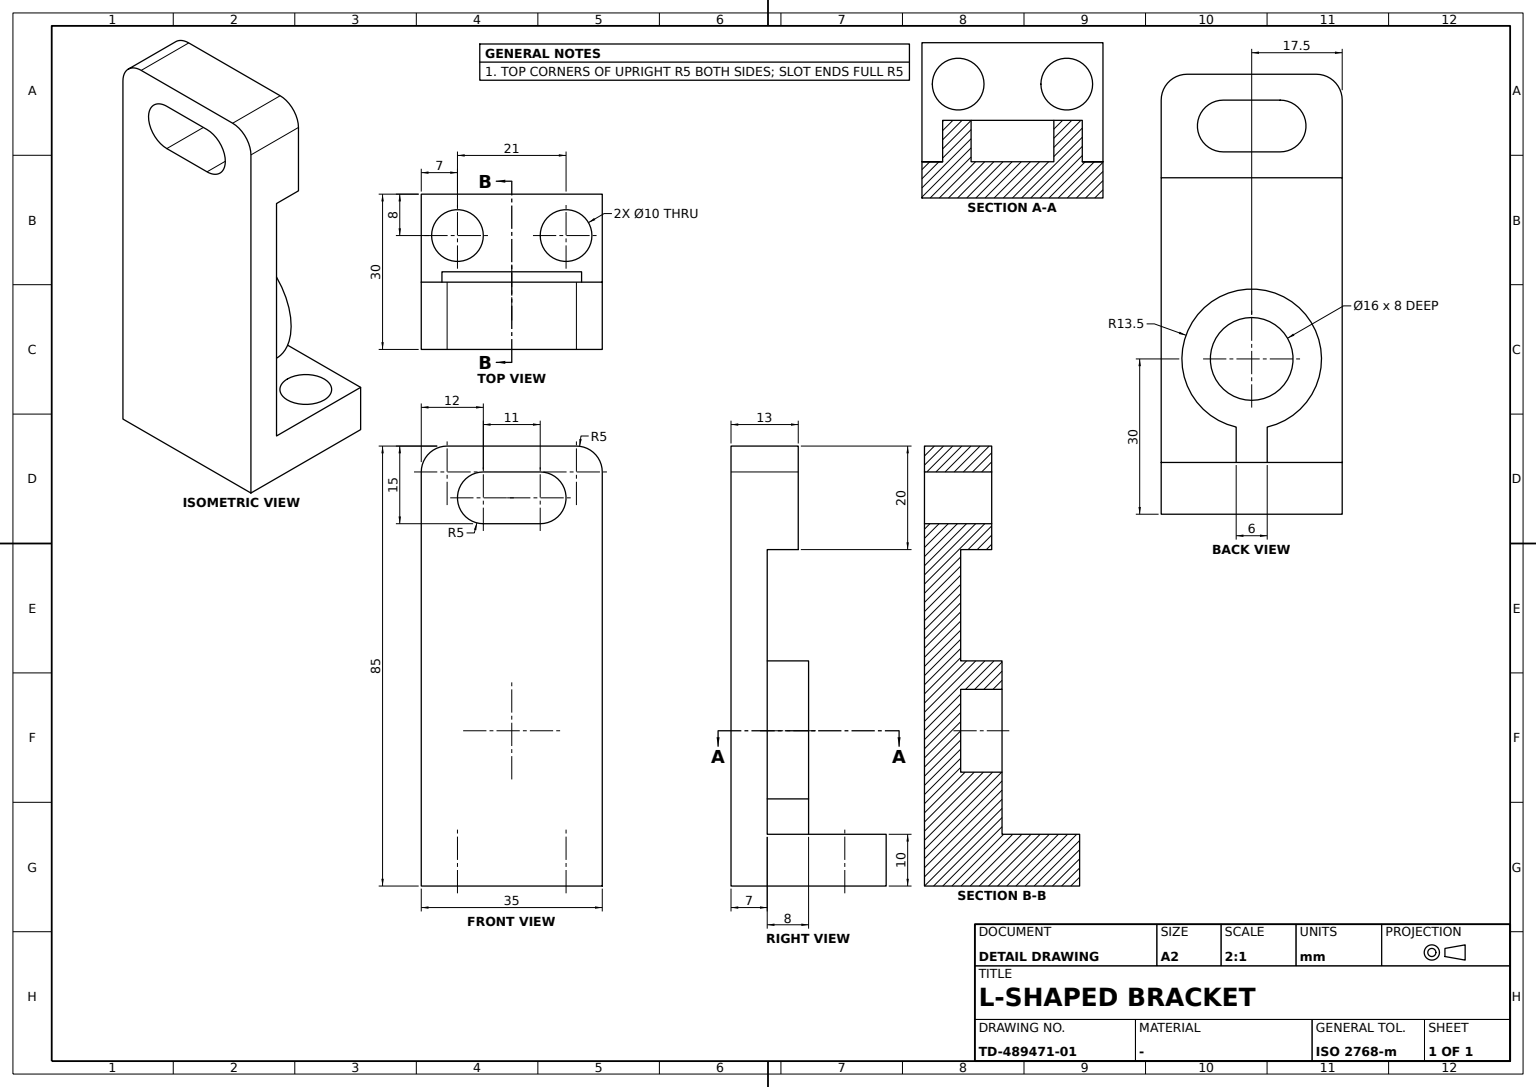
CATIA V5 part; units mm, degrees
sketch "Sketch1" plane through (0, 0, 0) normal (1, 0, 0) x (0, 1, 0)
  line L0 (0, 0) -> (0, 85)
  line L1 (0, 85) -> (13, 85)
  line L2 (13, 85) -> (13, 65)
  line L3 (13, 65) -> (7, 65)
  line L4 (7, 65) -> (7, 10)
  line L5 (7, 10) -> (30, 10)
  line L6 (30, 10) -> (30, 0)
  point P0 (30, 0)
  line L7 (30, 0) -> (0, 0)
  dimension "length L7" = 30
  dimension "length L6" = 10
  dimension "length L2" = 20
  dimension "distance L7 L1" = 85
  dimension "distance L2 L0" = 13
  dimension "distance L4 L0" = 7
  constraint vertical L0 y-axis
  constraint vertical L2 y-axis
  constraint vertical L4 y-axis
  constraint vertical L6 y-axis
  constraint horizontal L1 x-axis
  constraint horizontal L3 x-axis
  constraint horizontal L5 x-axis
  constraint horizontal L7 x-axis
  constraint coincidence P0 x-axis
extrude "Pad1" add sketch "Sketch1" along normal mid plane 35
fillet "Fillet1" radius 5 1 edges at (17.5, 6.5, 85)
fillet "Fillet2" radius 5 1 edges at (-17.5, 6.5, 85)
sketch "Sketch2" plane through (0, 0, 10) normal (0, 0, 1) x (0, 1, 0)
  circle A0 centre (22, 10.5) radius 5
  point P0 (22, 10.5)
  line L0 (30, 17.5) -> (7, 17.5) construction
  line L1 (30, 17.5) -> (30, -17.5) construction
  circle A1 centre (22, -10.5) radius 5
  dimension "radius A0" = 5
  dimension "distance L0 P0" = 7
  dimension "distance P0 L1" = 8
  constraint symmetry A0 A1 x-axis
extrude "Pocket1" cut sketch "Sketch2" against normal blind 17.5
sketch "Sketch3" plane through (0, 7, 0) normal (0, 1, 0) x (-1, 0, 0)
  arc A0 (3, 16.8376) -> (-3, 16.8376) centre (0, 30) ccw
  point P0 (0, 30)
  circle A1 centre (0, 30) radius 8
  line L0 (-3, 16.8376) -> (-3, 10)
  line L1 (-3, 10) -> (3, 10)
  line L2 (3, 10) -> (3, 16.8376)
  line L3 (17.5, 10) -> (-17.5, 10) construction
  dimension "radius A0" = 13.5
  dimension "radius A1" = 8
  dimension "distance P0 L1" = 20
  dimension "distance L0 L2" = 6
  constraint coincidence P0 y-axis
  constraint coincidence L1 L3
  constraint vertical L0 y-axis
  constraint vertical L2 y-axis
  constraint horizontal L1 x-axis
  constraint concentricity A1 A0
  constraint symmetry L0 L2 y-axis
extrude "Pad2" add sketch "Sketch3" along normal blind 8
sketch "Sketch4" plane through (0, 13, 0) normal (0, 1, 0) x (-1, 0, 0)
  arc A0 (-5.5, 80) -> (-5.5, 70) centre (-5.5, 75) ccw
  point P0 (-5.5, 75)
  arc A1 (5.5, 70) -> (5.5, 80) centre (5.5, 75) ccw
  point P1 (5.5, 75)
  line L0 (-5.5, 80) -> (5.5, 80)
  line L1 (17.5, 85) -> (-17.5, 85) construction
  line L2 (-5.5, 70) -> (5.5, 70)
  dimension "radius A1" = 5
  dimension "distance L0 L1" = 5
  dimension "distance P0 P1" = 11
  constraint horizontal L0 x-axis
  constraint horizontal L2 x-axis
  constraint tangency L2 A1
  constraint tangency A0 L2
  constraint tangency L0 A0
  constraint tangency L0 A1
  constraint symmetry A0 A1 y-axis
extrude "Pocket2" cut sketch "Sketch4" against normal up to next
